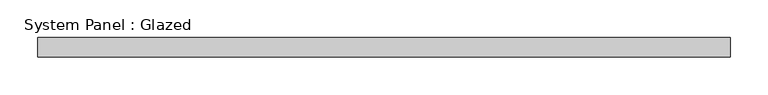
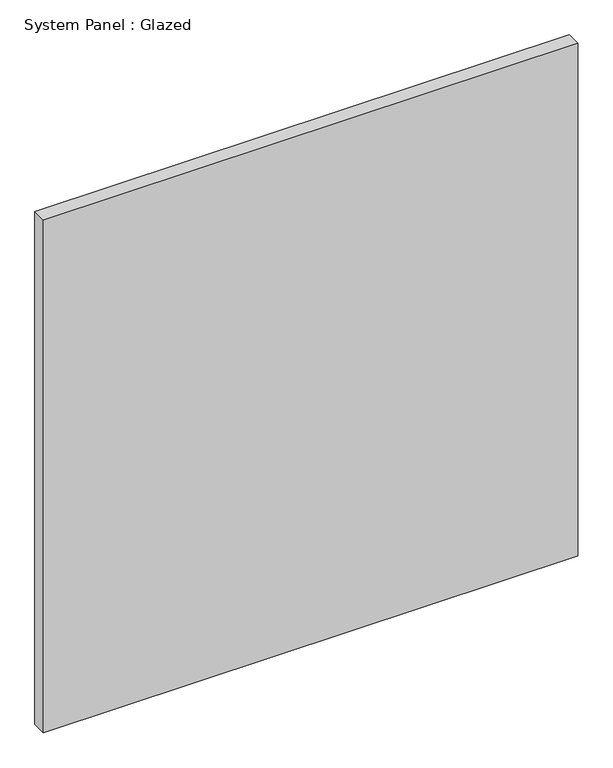
"""IFC4 building model written with IfcOpenShell, lengths in millimetres: plate geometry, System Panel : Glazed."""

from ifc_helpers import new_model, si_unit, origin, origin_with_axes, place, context, project, spatial, polyline, outline, extrude, source, transform, mapped, element, save


def system_panel_glazed_0a91d840(model_context):
    return source(origin(), model_context, "Body", "SweptSolid", [
        extrude(outline(polyline([(457.2, 19.05), (-457.2, 19.05), (-457.2, 44.45), (457.2, 44.45), (457.2, 19.05)])), origin_with_axes(), (0.0, 0.0, 1.0), 927.5610283),
    ])


if __name__ == "__main__":
    model = new_model("IFC4")
    model_context = context("Model", 3, world=origin())
    ifc_project = project(units=[si_unit("LENGTHUNIT", "METRE", prefix="MILLI")], contexts=[model_context])
    site = spatial("IfcSite", under=ifc_project)
    building = spatial("IfcBuilding", under=site)
    placement = place(None, origin())
    system_panel_glazed_shape = system_panel_glazed_0a91d840(model_context)
    element("IfcPlate", 1, ObjectType="System Panel : Glazed", at=placement, inside=building, context=model_context, shape_type="MappedRepresentation", body=[
        mapped(system_panel_glazed_shape, transform((0.0, 0.0, 0.0), x_axis=(1.0, 0.0, 0.0), y_axis=(0.0, 1.0, 0.0), z_axis=(0.0, 0.0, 1.0))),
    ])
    save(model, "model.ifc")

# Revit data of these elements
# Type "System Panel : Glazed"
#   Construction Type Id = "GSP4R"
#   Analytic Construction = "1/8 in Pilkington single glazing"
#   Visual Light Transmittance = 0.9
#   Solar Heat Gain Coefficient = 0.86
#   Heat Transfer Coefficient (U) = 1.18115 BTU/(h·ft²·°F)
# Element 1 (IfcPlate, "System Panel : Glazed")
#   Materials on its faces: "Glass"
# Materials
#   "Glass": class "Glass", colour RGB 0 128 192, transparency 0.75, Description = "Soda Lime Glass", Cost = 0
